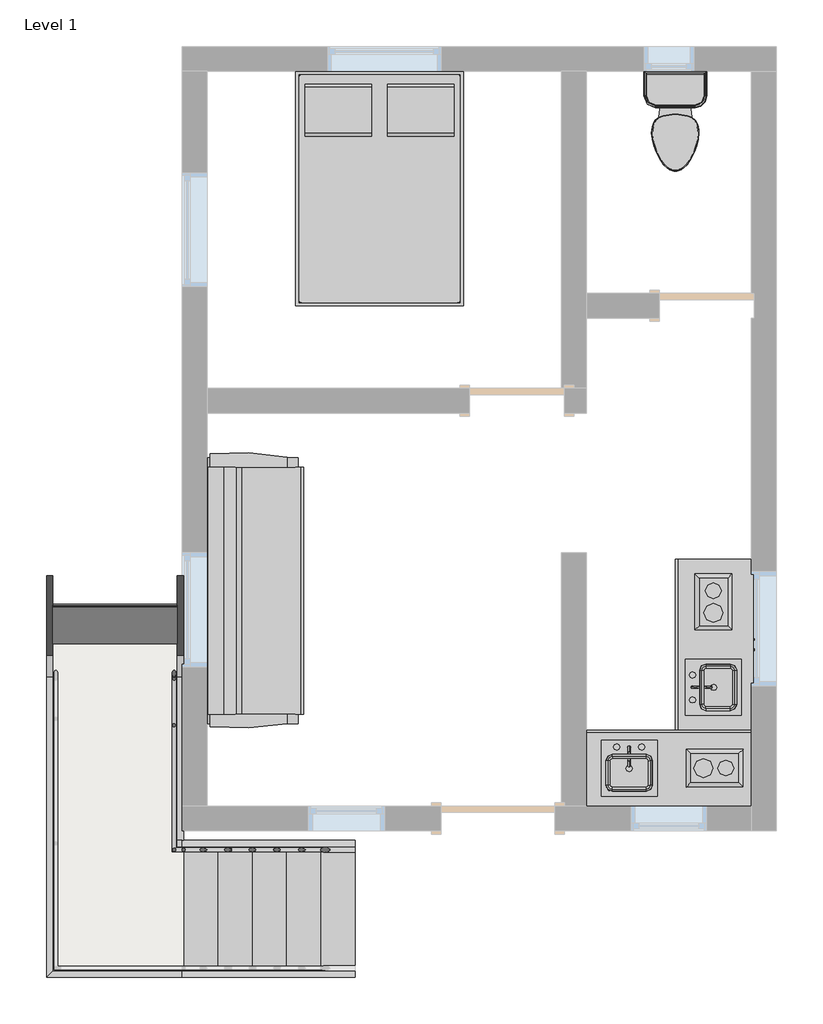
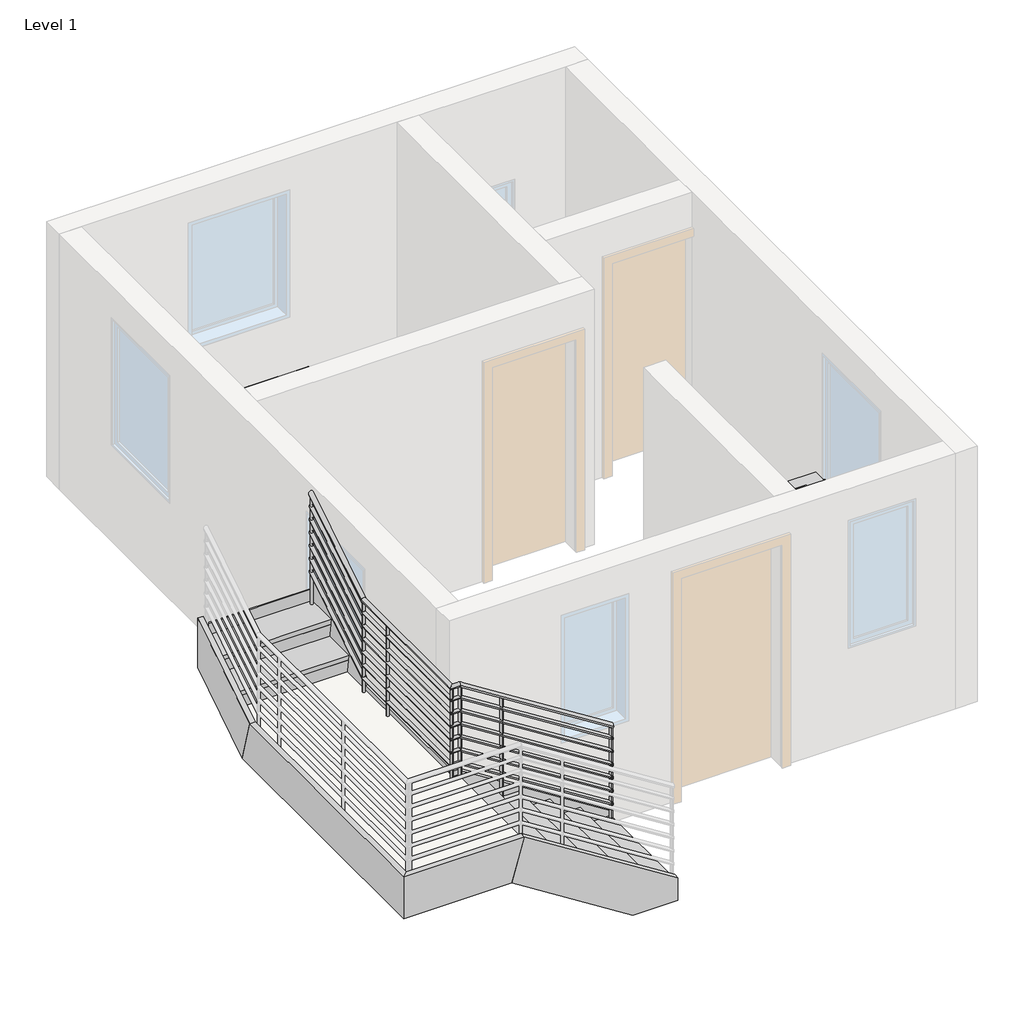
# One storey, part 3 of 3: 7 members, 4 furniture elements, 4 proxies, 3 flow terminals, 2 stair flights, 1 railing, 1 slab.
"""IFC4 building model written with IfcOpenShell, lengths in millimetres."""

from ifc_helpers import new_model, si_unit, point, frame, frame_2d, origin, place, context, project, spatial, polyline, circle_curve, ellipse_curve, trimmed, segment, composite_curve, outline, extrude, faceted_brep, transform, mapped, element, save
from ifc_brep_helpers import plane_surface, cylinder_surface, advanced_brep
from components import m_cook_top_2_unit_305_x_457mm_ebea1746, m_kitchenette_small_1372mm_f81b7602, m_sink_kitchen_island_450_x_450mm_f969cf2d, m_toilet_domestic_3d_m_toilet_domestic_3d_5cb52bd4, m_toilet_domestic_3d_m_toilet_domestic_3d_183bbd19, m_bed_box_1346_x_1880mm_double_b32eb57e, m_counter_top_w_sink_hole_600mm_depth_edbb3572, m_sofa_pensi_2134mm_91f3548c, non_monolithic_landing_de183352, stair_flight_50mm_tread_25mm_nosing_13mm_riser_1fd5534d, stair_flight_50mm_tread_25mm_nosing_13mm_riser_775a8025

model = new_model("IFC4")

# Units and contexts
model_context = context("Model", 3, world=origin())
ifc_project = project(units=[si_unit("LENGTHUNIT", "METRE", prefix="MILLI")], contexts=[model_context])

# Site, building, storey
site = spatial("IfcSite", under=ifc_project)
building = spatial("IfcBuilding", under=site)
storey = spatial("IfcBuildingStorey", under=building, Name="Level 1", Elevation=0.0)

# Proxies
placement = place(None, origin())
m_cook_top_2_unit_305_x_457mm_shape = m_cook_top_2_unit_305_x_457mm_ebea1746(model_context)
element("IfcBuildingElementProxy", 1, Name="M_Cook Top-2 Unit : 305 x 457mm", ObjectType="M_Cook Top-2 Unit : 305 x 457mm", at=placement, inside=storey, context=model_context, shape_type="MappedRepresentation", body=[
    mapped(m_cook_top_2_unit_305_x_457mm_shape, transform((-7256.3238606, 6264.0835626, 40.0), x_axis=(0.0, 1.0, 0.0), y_axis=(-1.0, 0.0, 0.0), z_axis=(0.0, 0.0, 1.0))),
])
element("IfcBuildingElementProxy", 2, Name="M_Cook Top-2 Unit : 305 x 457mm", ObjectType="M_Cook Top-2 Unit : 305 x 457mm", at=placement, inside=storey, context=model_context, shape_type="MappedRepresentation", body=[
    mapped(m_cook_top_2_unit_305_x_457mm_shape, transform((-7220.3486562, 7704.5083582, 40.0), x_axis=(-1.0000000000000002, 0.0, 0.0), y_axis=(0.0, -1.0000000000000002, 0.0), z_axis=(0.0, 0.0, 1.0))),
])
m_kitchenette_small_1372mm_shape = m_kitchenette_small_1372mm_f81b7602(model_context)
element("IfcBuildingElementProxy", 3, Name="M_Kitchenette - Small : 1372mm", ObjectType="M_Kitchenette - Small : 1372mm", at=placement, inside=storey, context=model_context, shape_type="MappedRepresentation", body=[
    mapped(m_kitchenette_small_1372mm_shape, transform((-7648.2863611, 6645.2835626, 0.0), x_axis=(1.0, 0.0, 0.0), y_axis=(0.0, 1.0, 0.0), z_axis=(0.0, 0.0, 1.0))),
])
element("IfcBuildingElementProxy", 4, Name="M_Kitchenette - Small : 1372mm", ObjectType="M_Kitchenette - Small : 1372mm", at=placement, inside=storey, context=model_context, shape_type="MappedRepresentation", body=[
    mapped(m_kitchenette_small_1372mm_shape, transform((-7601.5486562, 7312.5458577, 0.0), x_axis=(0.0, 1.0000000000000002, 0.0), y_axis=(-1.0000000000000002, 0.0, 0.0), z_axis=(0.0, 0.0, 1.0))),
])

# Flow terminals
m_sink_kitchen_island_450_x_450mm_shape = m_sink_kitchen_island_450_x_450mm_f969cf2d(model_context)
element("IfcFlowTerminal", 5, ObjectType="M_Sink Kitchen-Island : 450 x 450mm", at=placement, inside=storey, context=model_context, shape_type="MappedRepresentation", body=[
    mapped(m_sink_kitchen_island_450_x_450mm_shape, transform((-7988.2378968, 6337.9381615, 40.0), x_axis=(1.0, 0.0, 0.0), y_axis=(0.0, 1.0, 0.0), z_axis=(0.0, 0.0, 1.0))),
])
element("IfcFlowTerminal", 6, ObjectType="M_Sink Kitchen-Island : 450 x 450mm", at=placement, inside=storey, context=model_context, shape_type="MappedRepresentation", body=[
    mapped(m_sink_kitchen_island_450_x_450mm_shape, transform((-7294.2032551, 6972.5943221, 40.0), x_axis=(0.0, 1.0000000000000002, 0.0), y_axis=(-1.0000000000000002, 0.0, 0.0), z_axis=(0.0, 0.0, 1.0))),
])
m_toilet_domestic_3d_m_toilet_domestic_3d_shape = m_toilet_domestic_3d_m_toilet_domestic_3d_5cb52bd4(model_context)
m_toilet_domestic_3d_m_toilet_domestic_3d_2_shape = m_toilet_domestic_3d_m_toilet_domestic_3d_183bbd19(model_context)
element("IfcFlowTerminal", 7, ObjectType="M_Toilet-Domestic-3D : M_Toilet-Domestic-3D", at=placement, inside=storey, context=model_context, shape_type="MappedRepresentation", body=[
    mapped(m_toilet_domestic_3d_m_toilet_domestic_3d_shape, transform((-7602.1446836, 11436.5875353, 0.0), x_axis=(1.0, 0.0, 0.0), y_axis=(0.0, 1.0, 0.0), z_axis=(0.0, 0.0, 1.0))),
    mapped(m_toilet_domestic_3d_m_toilet_domestic_3d_2_shape, transform((-7602.1446836, 11436.5875353, 0.0), x_axis=(1.0, 0.0, 0.0), y_axis=(0.0, 1.0, 0.0), z_axis=(0.0, 0.0, 1.0))),
])

# Furniture
m_bed_box_1346_x_1880mm_double_shape = m_bed_box_1346_x_1880mm_double_b32eb57e(model_context)
element("IfcFurniture", 8, ObjectType="M_Bed-Box : 1346 x 1880mm - Double", at=placement, inside=storey, context=model_context, shape_type="MappedRepresentation", body=[
    mapped(m_bed_box_1346_x_1880mm_double_shape, transform((-10316.7011152, 11225.7130708, 0.0), x_axis=(1.0, 0.0, 0.0), y_axis=(0.0, 1.0, 0.0), z_axis=(0.0, 0.0, 1.0))),
])
m_counter_top_w_sink_hole_600mm_depth_shape = m_counter_top_w_sink_hole_600mm_depth_edbb3572(model_context)
element("IfcFurniture", 9, ObjectType="M_Counter Top w Sink Hole : 600mm Depth", at=placement, inside=storey, context=model_context, shape_type="MappedRepresentation", body=[
    mapped(m_counter_top_w_sink_hole_600mm_depth_shape, transform((-7115.0863611, 6645.2835626, 40.0), x_axis=(1.0, 0.0, 0.0), y_axis=(0.0, 1.0, 0.0), z_axis=(0.0, 0.0, 1.0))),
])
element("IfcFurniture", 10, ObjectType="M_Counter Top w Sink Hole : 600mm Depth", at=placement, inside=storey, context=model_context, shape_type="MappedRepresentation", body=[
    mapped(m_counter_top_w_sink_hole_600mm_depth_shape, transform((-7601.5486562, 7845.7458577, 40.0), x_axis=(0.0, 1.0000000000000002, 0.0), y_axis=(-1.0000000000000002, 0.0, 0.0), z_axis=(0.0, 0.0, 1.0))),
])
m_sofa_pensi_2134mm_shape = m_sofa_pensi_2134mm_91f3548c(model_context)
element("IfcFurniture", 11, ObjectType="M_Sofa-Pensi : 2134mm", at=placement, inside=storey, context=model_context, shape_type="MappedRepresentation", body=[
    mapped(m_sofa_pensi_2134mm_shape, transform((-10729.2388201, 7485.4773126, 0.0), x_axis=(0.0, 1.0, 0.0), y_axis=(-1.0, 0.0, 0.0), z_axis=(0.0, 0.0, 1.0))),
])

# Members
element("IfcMember", 12, ObjectType="Stringer - 50mm Width", at=placement, inside=storey, context=model_context, shape_type="SweptSolid", body=[
    extrude(outline(polyline([(0.0, -10176.2529994), (215.089535, -10176.2529994), (1090.8719878, -11561.084003), (690.8719878, -11676.953063), (0.0, -10584.5117322), (0.0, -10176.2529994)])), frame((0.0, 4659.8403022, 0.0), z_axis=(0.0, 1.0, 0.0), x_axis=(0.0, 0.0, 1.0)), (0.0, 0.0, 1.0), 50.0),
])
element("IfcMember", 13, ObjectType="Stringer - 50mm Width", at=placement, inside=storey, context=model_context, shape_type="SweptSolid", body=[
    extrude(outline(polyline([(0.0, -10176.2529994), (215.089535, -10176.2529994), (1090.8719878, -11561.084003), (1090.8719878, -11602.0529994), (643.5043587, -11602.0529994), (0.0, -10584.5117322), (0.0, -10176.2529994)])), frame((0.0, 5709.8660835, 0.0), z_axis=(0.0, 1.0, 0.0), x_axis=(0.0, 0.0, 1.0)), (0.0, 0.0, 1.0), 50.0),
])
element("IfcMember", 14, ObjectType="Stringer - 50mm Width", at=placement, inside=storey, context=model_context, shape_type="SweptSolid", body=[
    extrude(outline(polyline([(7184.5661471, 690.8719878), (7068.697087, 1090.8719878), (7883.8660835, 1606.3938828), (7883.8660835, 1133.1170069), (7184.5661471, 690.8719878)])), frame((-12652.0787807, 0.0, 0.0), z_axis=(1.0, 0.0, 0.0), x_axis=(0.0, 1.0, 0.0)), (0.0, 0.0, 1.0), 50.0),
])
element("IfcMember", 15, ObjectType="Stringer - 50mm Width", at=placement, inside=storey, context=model_context, shape_type="SweptSolid", body=[
    extrude(outline(polyline([(7184.5661471, 690.8719878), (7068.697087, 1090.8719878), (7883.8660835, 1606.3938828), (7883.8660835, 1133.1170069), (7184.5661471, 690.8719878)])), frame((-11602.0529994, 0.0, 0.0), z_axis=(1.0, 0.0, 0.0), x_axis=(0.0, 1.0, 0.0)), (0.0, 0.0, 1.0), 50.0),
])
element("IfcMember", 16, ObjectType="Stringer - 50mm Width", at=placement, inside=storey, context=model_context, shape_type="Brep", body=[
    faceted_brep([(-12602.0787807, 7068.697087, 1090.8719878), (-12652.0787807, 7068.697087, 1090.8719878), (-12652.0787807, 4659.8403022, 1090.8719878), (-12602.0787807, 4709.8403022, 1090.8719878), (-12602.0787807, 7184.5661471, 690.8719878), (-12602.0787807, 4709.8403022, 690.8719878), (-12652.0787807, 7184.5661471, 690.8719878), (-12652.0787807, 4659.8403022, 690.8719878)], [[[0, 1, 2, 3]], [[4, 0, 3, 5]], [[6, 4, 5, 7]], [[1, 6, 7, 2]], [[1, 0, 4, 6]], [[2, 7, 5, 3]]]),
])
element("IfcMember", 17, ObjectType="Stringer - 50mm Width", at=placement, inside=storey, context=model_context, shape_type="Brep", body=[
    faceted_brep([(-12602.0787807, 4709.8403022, 1090.8719878), (-12652.0787807, 4659.8403022, 1090.8719878), (-11561.084003, 4659.8403022, 1090.8719878), (-11561.084003, 4709.8403022, 1090.8719878), (-12602.0787807, 4709.8403022, 690.8719878), (-11676.953063, 4709.8403022, 690.8719878), (-12652.0787807, 4659.8403022, 690.8719878), (-11676.953063, 4659.8403022, 690.8719878)], [[[0, 1, 2, 3]], [[4, 0, 3, 5]], [[6, 4, 5, 7]], [[1, 6, 7, 2]], [[1, 0, 4, 6]], [[2, 7, 5, 3]]]),
])
element("IfcMember", 18, ObjectType="Stringer - 50mm Width", at=placement, inside=storey, context=model_context, shape_type="SweptSolid", body=[
    extrude(outline(polyline([(5759.8660835, 690.8719878), (5759.8660835, 1090.8719878), (7068.697087, 1090.8719878), (7184.5661471, 690.8719878), (5759.8660835, 690.8719878)])), frame((-11602.0529994, 0.0, 0.0), z_axis=(1.0, 0.0, 0.0), x_axis=(0.0, 1.0, 0.0)), (0.0, 0.0, 1.0), 50.0),
])

# Railing
element("IfcRailing", 19, ObjectType="900mm Pipe", at=placement, inside=storey, context=model_context, shape_type="SolidModel", body=[
    advanced_brep(
    [(-10176.2529994, 5704.4660835, 1050.2491997), (-10176.2529994, 5664.4660835, 1050.2491997), (-11557.0464524, 5704.4660835, 1923.4782609), (-11557.0464524, 5664.4660835, 1923.4782609), (-11607.4529994, 5704.4660835, 1923.4782609), (-11647.4529994, 5664.4660835, 1923.4782609), (-11607.4529994, 7064.6595365, 1923.4782609), (-11647.4529994, 7064.6595365, 1923.4782609), (-11607.4529994, 7883.8660835, 2441.5535475), (-11647.4529994, 7883.8660835, 2441.5535475)],
    [
        (0, 1, ellipse_curve(frame((-10176.2529994, 5684.4660835, 1050.2491997), z_axis=(1.0, 0.0, 0.0), x_axis=(0.0, 0.0, -1.0)), 23.6638438, 20.0)),
        (1, 0, ellipse_curve(frame((-10176.2529994, 5684.4660835, 1050.2491997), z_axis=(1.0, 0.0, 0.0), x_axis=(0.0, 0.0, -1.0)), 23.6638438, 20.0)),
        (0, 2),
        (2, 3, ellipse_curve(frame((-11557.0464524, 5684.4660835, 1923.4782609), z_axis=(0.9605132043335073, 0.0, -0.2782344053149754), x_axis=(-0.278234405314975, 0.0, -0.9605132043335074)), 20.822202, 20.0)),
        (3, 1),
        (3, 2, ellipse_curve(frame((-11557.0464524, 5684.4660835, 1923.4782609), z_axis=(0.9605132043335073, 0.0, -0.2782344053149754), x_axis=(-0.278234405314975, 0.0, -0.9605132043335074)), 20.822202, 20.0)),
        (2, 4),
        (4, 5, ellipse_curve(frame((-11627.4529994, 5684.4660835, 1923.4782609), z_axis=(0.7071067811865452, -0.7071067811865499, 0.0), x_axis=(0.7071067811865497, 0.7071067811865452, 0.0)), 28.2842712, 20.0)),
        (5, 3),
        (5, 4, ellipse_curve(frame((-11627.4529994, 5684.4660835, 1923.4782609), z_axis=(0.7071067811865452, -0.7071067811865499, 0.0), x_axis=(0.7071067811865497, 0.7071067811865452, 0.0)), 28.2842712, 20.0)),
        (4, 6),
        (6, 7, ellipse_curve(frame((-11627.4529994, 7064.6595365, 1923.4782609), z_axis=(0.0, -0.9605132043335063, -0.27823440531497884), x_axis=(0.0, -0.2782344053149792, 0.9605132043335064)), 20.822202, 20.0)),
        (7, 5),
        (7, 6, ellipse_curve(frame((-11627.4529994, 7064.6595365, 1923.4782609), z_axis=(0.0, -0.9605132043335063, -0.27823440531497884), x_axis=(0.0, -0.2782344053149792, 0.9605132043335064)), 20.822202, 20.0)),
        (8, 9, ellipse_curve(frame((-11627.4529994, 7883.8660835, 2441.5535475), z_axis=(0.0, 1.0, 0.0), x_axis=(0.0, 0.0, -1.0)), 23.6638438, 20.0)),
        (9, 8, ellipse_curve(frame((-11627.4529994, 7883.8660835, 2441.5535475), z_axis=(0.0, 1.0, 0.0), x_axis=(0.0, 0.0, -1.0)), 23.6638438, 20.0)),
        (6, 8),
        (9, 7),
    ],
    [
        plane_surface(frame((-10176.2529994, 5684.4660835, 1073.9130435), z_axis=(1.0, 0.0, 0.0), x_axis=(0.0, -1.0, 0.0))),
        cylinder_surface(frame((-10186.9429122, 5684.4660835, 1057.0096189), z_axis=(0.845171231398044, 0.0, -0.5344956404098298), x_axis=(0.0, -1.0, 0.0)), 20.0),
        cylinder_surface(frame((-11551.2529994, 5684.4660835, 1923.4782609), z_axis=(1.0, 0.0, 0.0), x_axis=(0.0, -1.0, 0.0)), 20.0),
        cylinder_surface(frame((-11627.4529994, 5684.4660835, 1923.4782609), z_axis=(0.0, -1.0, 0.0), x_axis=(-1.0, 0.0, 0.0)), 20.0),
        plane_surface(frame((-11627.4529994, 7883.8660835, 2465.2173913), z_axis=(0.0, 1.0, 0.0), x_axis=(0.0, 0.0, 1.0))),
        cylinder_surface(frame((-11627.4529994, 7069.5559963, 1926.5748362), z_axis=(0.0, -0.8451712313980402, -0.5344956404098358), x_axis=(-1.0, 0.0, 0.0)), 20.0),
    ],
    [
        (0, [[1, 2]]),
        (1, [[-1, 3, 4, 5]]),
        (1, [[-2, -5, 6, -3]]),
        (2, [[-4, 7, 8, 9]]),
        (2, [[-6, -9, 10, -7]]),
        (3, [[-8, 11, 12, 13]]),
        (3, [[-10, -13, 14, -11]]),
        (4, [[15, 16]]),
        (5, [[-12, 17, -16, 18]]),
        (5, [[-14, -18, -15, -17]]),
    ],
),
    advanced_brep(
    [(-10176.2529994, 5669.4660835, 931.1651606), (-10176.2529994, 5699.4660835, 931.1651606), (-11555.5980892, 5669.4660835, 1803.4782609), (-11555.5980892, 5699.4660835, 1803.4782609), (-11642.4529994, 5669.4660835, 1803.4782609), (-11612.4529994, 5699.4660835, 1803.4782609), (-11642.4529994, 7063.2111733, 1803.4782609), (-11612.4529994, 7063.2111733, 1803.4782609), (-11642.4529994, 7883.8660835, 2322.4695085), (-11612.4529994, 7883.8660835, 2322.4695085)],
    [
        (0, 1, ellipse_curve(frame((-10176.2529994, 5684.4660835, 931.1651606), z_axis=(1.0, 0.0, 0.0), x_axis=(0.0, 0.0, -1.0)), 17.7478828, 15.0)),
        (1, 0, ellipse_curve(frame((-10176.2529994, 5684.4660835, 931.1651606), z_axis=(1.0, 0.0, 0.0), x_axis=(0.0, 0.0, -1.0)), 17.7478828, 15.0)),
        (0, 2),
        (2, 3, ellipse_curve(frame((-11555.5980892, 5684.4660835, 1803.4782609), z_axis=(0.9605132043335073, 0.0, -0.27823440531497534), x_axis=(-0.27823440531497506, 0.0, -0.9605132043335075)), 15.6166515, 15.0)),
        (3, 1),
        (3, 2, ellipse_curve(frame((-11555.5980892, 5684.4660835, 1803.4782609), z_axis=(0.9605132043335073, 0.0, -0.27823440531497534), x_axis=(-0.27823440531497506, 0.0, -0.9605132043335075)), 15.6166515, 15.0)),
        (2, 4),
        (4, 5, ellipse_curve(frame((-11627.4529994, 5684.4660835, 1803.4782609), z_axis=(0.7071067811865452, -0.7071067811865499, 0.0), x_axis=(0.7071067811865497, 0.7071067811865452, 0.0)), 21.2132034, 15.0)),
        (5, 3),
        (5, 4, ellipse_curve(frame((-11627.4529994, 5684.4660835, 1803.4782609), z_axis=(0.7071067811865452, -0.7071067811865499, 0.0), x_axis=(0.7071067811865497, 0.7071067811865452, 0.0)), 21.2132034, 15.0)),
        (4, 6),
        (6, 7, ellipse_curve(frame((-11627.4529994, 7063.2111733, 1803.4782609), z_axis=(0.0, -0.9605132043335064, -0.2782344053149787), x_axis=(0.0, -0.27823440531497856, 0.9605132043335064)), 15.6166515, 15.0)),
        (7, 5),
        (7, 6, ellipse_curve(frame((-11627.4529994, 7063.2111733, 1803.4782609), z_axis=(0.0, -0.9605132043335064, -0.2782344053149787), x_axis=(0.0, -0.27823440531497856, 0.9605132043335064)), 15.6166515, 15.0)),
        (8, 9, ellipse_curve(frame((-11627.4529994, 7883.8660835, 2322.4695085), z_axis=(0.0, 1.0, 0.0), x_axis=(0.0, 0.0, -1.0)), 17.7478828, 15.0)),
        (9, 8, ellipse_curve(frame((-11627.4529994, 7883.8660835, 2322.4695085), z_axis=(0.0, 1.0, 0.0), x_axis=(0.0, 0.0, -1.0)), 17.7478828, 15.0)),
        (6, 8),
        (9, 7),
    ],
    [
        plane_surface(frame((-10176.2529994, 5684.4660835, 948.9130435), z_axis=(1.0, 0.0, 0.0), x_axis=(0.0, -1.0, 0.0))),
        cylinder_surface(frame((-10184.270434, 5684.4660835, 936.235475), z_axis=(0.845171231398044, 0.0, -0.5344956404098297), x_axis=(0.0, 1.0, 0.0)), 15.0),
        cylinder_surface(frame((-11551.2529994, 5684.4660835, 1803.4782609), z_axis=(1.0, 0.0, 0.0), x_axis=(0.0, 1.0, 0.0)), 15.0),
        cylinder_surface(frame((-11627.4529994, 5684.4660835, 1803.4782609), z_axis=(0.0, -1.0, 0.0), x_axis=(1.0, 0.0, 0.0)), 15.0),
        plane_surface(frame((-11627.4529994, 7883.8660835, 2340.2173913), z_axis=(0.0, 1.0, 0.0), x_axis=(0.0, 0.0, 1.0))),
        cylinder_surface(frame((-11627.4529994, 7066.8835181, 1805.8006924), z_axis=(0.0, -0.8451712313980403, -0.5344956404098355), x_axis=(1.0, 0.0, 0.0)), 15.0),
    ],
    [
        (0, [[1, 2]]),
        (1, [[-1, 3, 4, 5]]),
        (1, [[-2, -5, 6, -3]]),
        (2, [[-4, 7, 8, 9]]),
        (2, [[-6, -9, 10, -7]]),
        (3, [[-8, 11, 12, 13]]),
        (3, [[-10, -13, 14, -11]]),
        (4, [[15, 16]]),
        (5, [[-12, 17, -16, 18]]),
        (5, [[-14, -18, -15, -17]]),
    ],
),
    advanced_brep(
    [(-10176.2529994, 5669.4660835, 806.1651606), (-10176.2529994, 5699.4660835, 806.1651606), (-11555.5980892, 5669.4660835, 1678.4782609), (-11555.5980892, 5699.4660835, 1678.4782609), (-11642.4529994, 5669.4660835, 1678.4782609), (-11612.4529994, 5699.4660835, 1678.4782609), (-11642.4529994, 7063.2111733, 1678.4782609), (-11612.4529994, 7063.2111733, 1678.4782609), (-11642.4529994, 7883.8660835, 2197.4695085), (-11612.4529994, 7883.8660835, 2197.4695085)],
    [
        (0, 1, ellipse_curve(frame((-10176.2529994, 5684.4660835, 806.1651606), z_axis=(1.0, 0.0, 0.0), x_axis=(0.0, 0.0, -1.0)), 17.7478828, 15.0)),
        (1, 0, ellipse_curve(frame((-10176.2529994, 5684.4660835, 806.1651606), z_axis=(1.0, 0.0, 0.0), x_axis=(0.0, 0.0, -1.0)), 17.7478828, 15.0)),
        (0, 2),
        (2, 3, ellipse_curve(frame((-11555.5980892, 5684.4660835, 1678.4782609), z_axis=(0.9605132043335073, 0.0, -0.27823440531497534), x_axis=(-0.27823440531497506, 0.0, -0.9605132043335075)), 15.6166515, 15.0)),
        (3, 1),
        (3, 2, ellipse_curve(frame((-11555.5980892, 5684.4660835, 1678.4782609), z_axis=(0.9605132043335073, 0.0, -0.27823440531497534), x_axis=(-0.27823440531497506, 0.0, -0.9605132043335075)), 15.6166515, 15.0)),
        (2, 4),
        (4, 5, ellipse_curve(frame((-11627.4529994, 5684.4660835, 1678.4782609), z_axis=(0.7071067811865452, -0.7071067811865499, 0.0), x_axis=(0.7071067811865497, 0.7071067811865452, 0.0)), 21.2132034, 15.0)),
        (5, 3),
        (5, 4, ellipse_curve(frame((-11627.4529994, 5684.4660835, 1678.4782609), z_axis=(0.7071067811865452, -0.7071067811865499, 0.0), x_axis=(0.7071067811865497, 0.7071067811865452, 0.0)), 21.2132034, 15.0)),
        (4, 6),
        (6, 7, ellipse_curve(frame((-11627.4529994, 7063.2111733, 1678.4782609), z_axis=(0.0, -0.9605132043335063, -0.27823440531497884), x_axis=(0.0, -0.2782344053149792, 0.9605132043335064)), 15.6166515, 15.0)),
        (7, 5),
        (7, 6, ellipse_curve(frame((-11627.4529994, 7063.2111733, 1678.4782609), z_axis=(0.0, -0.9605132043335063, -0.27823440531497884), x_axis=(0.0, -0.2782344053149792, 0.9605132043335064)), 15.6166515, 15.0)),
        (8, 9, ellipse_curve(frame((-11627.4529994, 7883.8660835, 2197.4695085), z_axis=(0.0, 1.0, 0.0), x_axis=(0.0, 0.0, -1.0)), 17.7478828, 15.0)),
        (9, 8, ellipse_curve(frame((-11627.4529994, 7883.8660835, 2197.4695085), z_axis=(0.0, 1.0, 0.0), x_axis=(0.0, 0.0, -1.0)), 17.7478828, 15.0)),
        (6, 8),
        (9, 7),
    ],
    [
        plane_surface(frame((-10176.2529994, 5684.4660835, 823.9130435), z_axis=(1.0, 0.0, 0.0), x_axis=(0.0, -1.0, 0.0))),
        cylinder_surface(frame((-10184.270434, 5684.4660835, 811.235475), z_axis=(0.845171231398044, 0.0, -0.5344956404098297), x_axis=(0.0, 1.0, 0.0)), 15.0),
        cylinder_surface(frame((-11551.2529994, 5684.4660835, 1678.4782609), z_axis=(1.0, 0.0, 0.0), x_axis=(0.0, 1.0, 0.0)), 15.0),
        cylinder_surface(frame((-11627.4529994, 5684.4660835, 1678.4782609), z_axis=(0.0, -1.0, 0.0), x_axis=(1.0, 0.0, 0.0)), 15.0),
        plane_surface(frame((-11627.4529994, 7883.8660835, 2215.2173913), z_axis=(0.0, 1.0, 0.0), x_axis=(0.0, 0.0, 1.0))),
        cylinder_surface(frame((-11627.4529994, 7066.8835181, 1680.8006924), z_axis=(0.0, -0.8451712313980402, -0.5344956404098358), x_axis=(1.0, 0.0, 0.0)), 15.0),
    ],
    [
        (0, [[1, 2]]),
        (1, [[-1, 3, 4, 5]]),
        (1, [[-2, -5, 6, -3]]),
        (2, [[-4, 7, 8, 9]]),
        (2, [[-6, -9, 10, -7]]),
        (3, [[-8, 11, 12, 13]]),
        (3, [[-10, -13, 14, -11]]),
        (4, [[15, 16]]),
        (5, [[-12, 17, -16, 18]]),
        (5, [[-14, -18, -15, -17]]),
    ],
),
    advanced_brep(
    [(-10176.2529994, 5669.4660835, 681.1651606), (-10176.2529994, 5699.4660835, 681.1651606), (-11555.5980892, 5669.4660835, 1553.4782609), (-11555.5980892, 5699.4660835, 1553.4782609), (-11642.4529994, 5669.4660835, 1553.4782609), (-11612.4529994, 5699.4660835, 1553.4782609), (-11642.4529994, 7063.2111733, 1553.4782609), (-11612.4529994, 7063.2111733, 1553.4782609), (-11642.4529994, 7883.8660835, 2072.4695085), (-11612.4529994, 7883.8660835, 2072.4695085)],
    [
        (0, 1, ellipse_curve(frame((-10176.2529994, 5684.4660835, 681.1651606), z_axis=(1.0, 0.0, 0.0), x_axis=(0.0, 0.0, -1.0)), 17.7478828, 15.0)),
        (1, 0, ellipse_curve(frame((-10176.2529994, 5684.4660835, 681.1651606), z_axis=(1.0, 0.0, 0.0), x_axis=(0.0, 0.0, -1.0)), 17.7478828, 15.0)),
        (0, 2),
        (2, 3, ellipse_curve(frame((-11555.5980892, 5684.4660835, 1553.4782609), z_axis=(0.9605132043335073, 0.0, -0.27823440531497534), x_axis=(-0.27823440531497506, 0.0, -0.9605132043335075)), 15.6166515, 15.0)),
        (3, 1),
        (3, 2, ellipse_curve(frame((-11555.5980892, 5684.4660835, 1553.4782609), z_axis=(0.9605132043335073, 0.0, -0.27823440531497534), x_axis=(-0.27823440531497506, 0.0, -0.9605132043335075)), 15.6166515, 15.0)),
        (2, 4),
        (4, 5, ellipse_curve(frame((-11627.4529994, 5684.4660835, 1553.4782609), z_axis=(0.7071067811865452, -0.7071067811865499, 0.0), x_axis=(0.7071067811865497, 0.7071067811865452, 0.0)), 21.2132034, 15.0)),
        (5, 3),
        (5, 4, ellipse_curve(frame((-11627.4529994, 5684.4660835, 1553.4782609), z_axis=(0.7071067811865452, -0.7071067811865499, 0.0), x_axis=(0.7071067811865497, 0.7071067811865452, 0.0)), 21.2132034, 15.0)),
        (4, 6),
        (6, 7, ellipse_curve(frame((-11627.4529994, 7063.2111733, 1553.4782609), z_axis=(0.0, -0.9605132043335064, -0.2782344053149787), x_axis=(0.0, -0.27823440531497856, 0.9605132043335064)), 15.6166515, 15.0)),
        (7, 5),
        (7, 6, ellipse_curve(frame((-11627.4529994, 7063.2111733, 1553.4782609), z_axis=(0.0, -0.9605132043335064, -0.2782344053149787), x_axis=(0.0, -0.27823440531497856, 0.9605132043335064)), 15.6166515, 15.0)),
        (8, 9, ellipse_curve(frame((-11627.4529994, 7883.8660835, 2072.4695085), z_axis=(0.0, 1.0, 0.0), x_axis=(0.0, 0.0, -1.0)), 17.7478828, 15.0)),
        (9, 8, ellipse_curve(frame((-11627.4529994, 7883.8660835, 2072.4695085), z_axis=(0.0, 1.0, 0.0), x_axis=(0.0, 0.0, -1.0)), 17.7478828, 15.0)),
        (6, 8),
        (9, 7),
    ],
    [
        plane_surface(frame((-10176.2529994, 5684.4660835, 698.9130435), z_axis=(1.0, 0.0, 0.0), x_axis=(0.0, -1.0, 0.0))),
        cylinder_surface(frame((-10184.270434, 5684.4660835, 686.235475), z_axis=(0.845171231398044, 0.0, -0.5344956404098297), x_axis=(0.0, 1.0, 0.0)), 15.0),
        cylinder_surface(frame((-11551.2529994, 5684.4660835, 1553.4782609), z_axis=(1.0, 0.0, 0.0), x_axis=(0.0, 1.0, 0.0)), 15.0),
        cylinder_surface(frame((-11627.4529994, 5684.4660835, 1553.4782609), z_axis=(0.0, -1.0, 0.0), x_axis=(1.0, 0.0, 0.0)), 15.0),
        plane_surface(frame((-11627.4529994, 7883.8660835, 2090.2173913), z_axis=(0.0, 1.0, 0.0), x_axis=(0.0, 0.0, 1.0))),
        cylinder_surface(frame((-11627.4529994, 7066.8835181, 1555.8006924), z_axis=(0.0, -0.8451712313980403, -0.5344956404098355), x_axis=(1.0, 0.0, 0.0)), 15.0),
    ],
    [
        (0, [[1, 2]]),
        (1, [[-1, 3, 4, 5]]),
        (1, [[-2, -5, 6, -3]]),
        (2, [[-4, 7, 8, 9]]),
        (2, [[-6, -9, 10, -7]]),
        (3, [[-8, 11, 12, 13]]),
        (3, [[-10, -13, 14, -11]]),
        (4, [[15, 16]]),
        (5, [[-12, 17, -16, 18]]),
        (5, [[-14, -18, -15, -17]]),
    ],
),
    advanced_brep(
    [(-10176.2529994, 5669.4660835, 556.1651606), (-10176.2529994, 5699.4660835, 556.1651606), (-11555.5980892, 5669.4660835, 1428.4782609), (-11555.5980892, 5699.4660835, 1428.4782609), (-11642.4529994, 5669.4660835, 1428.4782609), (-11612.4529994, 5699.4660835, 1428.4782609), (-11642.4529994, 7063.2111733, 1428.4782609), (-11612.4529994, 7063.2111733, 1428.4782609), (-11642.4529994, 7883.8660835, 1947.4695085), (-11612.4529994, 7883.8660835, 1947.4695085)],
    [
        (0, 1, ellipse_curve(frame((-10176.2529994, 5684.4660835, 556.1651606), z_axis=(1.0, 0.0, 0.0), x_axis=(0.0, 0.0, -1.0)), 17.7478828, 15.0)),
        (1, 0, ellipse_curve(frame((-10176.2529994, 5684.4660835, 556.1651606), z_axis=(1.0, 0.0, 0.0), x_axis=(0.0, 0.0, -1.0)), 17.7478828, 15.0)),
        (0, 2),
        (2, 3, ellipse_curve(frame((-11555.5980892, 5684.4660835, 1428.4782609), z_axis=(0.9605132043335073, 0.0, -0.27823440531497534), x_axis=(-0.27823440531497506, 0.0, -0.9605132043335075)), 15.6166515, 15.0)),
        (3, 1),
        (3, 2, ellipse_curve(frame((-11555.5980892, 5684.4660835, 1428.4782609), z_axis=(0.9605132043335073, 0.0, -0.27823440531497534), x_axis=(-0.27823440531497506, 0.0, -0.9605132043335075)), 15.6166515, 15.0)),
        (2, 4),
        (4, 5, ellipse_curve(frame((-11627.4529994, 5684.4660835, 1428.4782609), z_axis=(0.7071067811865452, -0.7071067811865499, 0.0), x_axis=(0.7071067811865497, 0.7071067811865452, 0.0)), 21.2132034, 15.0)),
        (5, 3),
        (5, 4, ellipse_curve(frame((-11627.4529994, 5684.4660835, 1428.4782609), z_axis=(0.7071067811865452, -0.7071067811865499, 0.0), x_axis=(0.7071067811865497, 0.7071067811865452, 0.0)), 21.2132034, 15.0)),
        (4, 6),
        (6, 7, ellipse_curve(frame((-11627.4529994, 7063.2111733, 1428.4782609), z_axis=(0.0, -0.9605132043335063, -0.27823440531497884), x_axis=(0.0, -0.2782344053149792, 0.9605132043335064)), 15.6166515, 15.0)),
        (7, 5),
        (7, 6, ellipse_curve(frame((-11627.4529994, 7063.2111733, 1428.4782609), z_axis=(0.0, -0.9605132043335063, -0.27823440531497884), x_axis=(0.0, -0.2782344053149792, 0.9605132043335064)), 15.6166515, 15.0)),
        (8, 9, ellipse_curve(frame((-11627.4529994, 7883.8660835, 1947.4695085), z_axis=(0.0, 1.0, 0.0), x_axis=(0.0, 0.0, -1.0)), 17.7478828, 15.0)),
        (9, 8, ellipse_curve(frame((-11627.4529994, 7883.8660835, 1947.4695085), z_axis=(0.0, 1.0, 0.0), x_axis=(0.0, 0.0, -1.0)), 17.7478828, 15.0)),
        (6, 8),
        (9, 7),
    ],
    [
        plane_surface(frame((-10176.2529994, 5684.4660835, 573.9130435), z_axis=(1.0, 0.0, 0.0), x_axis=(0.0, -1.0, 0.0))),
        cylinder_surface(frame((-10184.270434, 5684.4660835, 561.235475), z_axis=(0.845171231398044, 0.0, -0.5344956404098297), x_axis=(0.0, 1.0, 0.0)), 15.0),
        cylinder_surface(frame((-11551.2529994, 5684.4660835, 1428.4782609), z_axis=(1.0, 0.0, 0.0), x_axis=(0.0, 1.0, 0.0)), 15.0),
        cylinder_surface(frame((-11627.4529994, 5684.4660835, 1428.4782609), z_axis=(0.0, -1.0, 0.0), x_axis=(1.0, 0.0, 0.0)), 15.0),
        plane_surface(frame((-11627.4529994, 7883.8660835, 1965.2173913), z_axis=(0.0, 1.0, 0.0), x_axis=(0.0, 0.0, 1.0))),
        cylinder_surface(frame((-11627.4529994, 7066.8835181, 1430.8006924), z_axis=(0.0, -0.8451712313980402, -0.5344956404098358), x_axis=(1.0, 0.0, 0.0)), 15.0),
    ],
    [
        (0, [[1, 2]]),
        (1, [[-1, 3, 4, 5]]),
        (1, [[-2, -5, 6, -3]]),
        (2, [[-4, 7, 8, 9]]),
        (2, [[-6, -9, 10, -7]]),
        (3, [[-8, 11, 12, 13]]),
        (3, [[-10, -13, 14, -11]]),
        (4, [[15, 16]]),
        (5, [[-12, 17, -16, 18]]),
        (5, [[-14, -18, -15, -17]]),
    ],
),
    advanced_brep(
    [(-10176.2529994, 5669.4660835, 431.1651606), (-10176.2529994, 5699.4660835, 431.1651606), (-11555.5980892, 5669.4660835, 1303.4782609), (-11555.5980892, 5699.4660835, 1303.4782609), (-11642.4529994, 5669.4660835, 1303.4782609), (-11612.4529994, 5699.4660835, 1303.4782609), (-11642.4529994, 7063.2111733, 1303.4782609), (-11612.4529994, 7063.2111733, 1303.4782609), (-11642.4529994, 7883.8660835, 1822.4695085), (-11612.4529994, 7883.8660835, 1822.4695085)],
    [
        (0, 1, ellipse_curve(frame((-10176.2529994, 5684.4660835, 431.1651606), z_axis=(1.0, 0.0, 0.0), x_axis=(0.0, 0.0, -1.0)), 17.7478828, 15.0)),
        (1, 0, ellipse_curve(frame((-10176.2529994, 5684.4660835, 431.1651606), z_axis=(1.0, 0.0, 0.0), x_axis=(0.0, 0.0, -1.0)), 17.7478828, 15.0)),
        (0, 2),
        (2, 3, ellipse_curve(frame((-11555.5980892, 5684.4660835, 1303.4782609), z_axis=(0.9605132043335073, 0.0, -0.27823440531497534), x_axis=(-0.27823440531497506, 0.0, -0.9605132043335075)), 15.6166515, 15.0)),
        (3, 1),
        (3, 2, ellipse_curve(frame((-11555.5980892, 5684.4660835, 1303.4782609), z_axis=(0.9605132043335073, 0.0, -0.27823440531497534), x_axis=(-0.27823440531497506, 0.0, -0.9605132043335075)), 15.6166515, 15.0)),
        (2, 4),
        (4, 5, ellipse_curve(frame((-11627.4529994, 5684.4660835, 1303.4782609), z_axis=(0.7071067811865452, -0.7071067811865499, 0.0), x_axis=(0.7071067811865497, 0.7071067811865452, 0.0)), 21.2132034, 15.0)),
        (5, 3),
        (5, 4, ellipse_curve(frame((-11627.4529994, 5684.4660835, 1303.4782609), z_axis=(0.7071067811865452, -0.7071067811865499, 0.0), x_axis=(0.7071067811865497, 0.7071067811865452, 0.0)), 21.2132034, 15.0)),
        (4, 6),
        (6, 7, ellipse_curve(frame((-11627.4529994, 7063.2111733, 1303.4782609), z_axis=(0.0, -0.9605132043335064, -0.2782344053149787), x_axis=(0.0, -0.27823440531497856, 0.9605132043335064)), 15.6166515, 15.0)),
        (7, 5),
        (7, 6, ellipse_curve(frame((-11627.4529994, 7063.2111733, 1303.4782609), z_axis=(0.0, -0.9605132043335064, -0.2782344053149787), x_axis=(0.0, -0.27823440531497856, 0.9605132043335064)), 15.6166515, 15.0)),
        (8, 9, ellipse_curve(frame((-11627.4529994, 7883.8660835, 1822.4695085), z_axis=(0.0, 1.0, 0.0), x_axis=(0.0, 0.0, -1.0)), 17.7478828, 15.0)),
        (9, 8, ellipse_curve(frame((-11627.4529994, 7883.8660835, 1822.4695085), z_axis=(0.0, 1.0, 0.0), x_axis=(0.0, 0.0, -1.0)), 17.7478828, 15.0)),
        (6, 8),
        (9, 7),
    ],
    [
        plane_surface(frame((-10176.2529994, 5684.4660835, 448.9130435), z_axis=(1.0, 0.0, 0.0), x_axis=(0.0, -1.0, 0.0))),
        cylinder_surface(frame((-10184.270434, 5684.4660835, 436.235475), z_axis=(0.845171231398044, 0.0, -0.5344956404098297), x_axis=(0.0, 1.0, 0.0)), 15.0),
        cylinder_surface(frame((-11551.2529994, 5684.4660835, 1303.4782609), z_axis=(1.0, 0.0, 0.0), x_axis=(0.0, 1.0, 0.0)), 15.0),
        cylinder_surface(frame((-11627.4529994, 5684.4660835, 1303.4782609), z_axis=(0.0, -1.0, 0.0), x_axis=(1.0, 0.0, 0.0)), 15.0),
        plane_surface(frame((-11627.4529994, 7883.8660835, 1840.2173913), z_axis=(0.0, 1.0, 0.0), x_axis=(0.0, 0.0, 1.0))),
        cylinder_surface(frame((-11627.4529994, 7066.8835181, 1305.8006924), z_axis=(0.0, -0.8451712313980403, -0.5344956404098355), x_axis=(1.0, 0.0, 0.0)), 15.0),
    ],
    [
        (0, [[1, 2]]),
        (1, [[-1, 3, 4, 5]]),
        (1, [[-2, -5, 6, -3]]),
        (2, [[-4, 7, 8, 9]]),
        (2, [[-6, -9, 10, -7]]),
        (3, [[-8, 11, 12, 13]]),
        (3, [[-10, -13, 14, -11]]),
        (4, [[15, 16]]),
        (5, [[-12, 17, -16, 18]]),
        (5, [[-14, -18, -15, -17]]),
    ],
),
    advanced_brep(
    [(-10176.2529994, 5669.4660835, 306.1651606), (-10176.2529994, 5699.4660835, 306.1651606), (-11555.5980892, 5669.4660835, 1178.4782609), (-11555.5980892, 5699.4660835, 1178.4782609), (-11642.4529994, 5669.4660835, 1178.4782609), (-11612.4529994, 5699.4660835, 1178.4782609), (-11642.4529994, 7063.2111733, 1178.4782609), (-11612.4529994, 7063.2111733, 1178.4782609), (-11642.4529994, 7883.8660835, 1697.4695085), (-11612.4529994, 7883.8660835, 1697.4695085)],
    [
        (0, 1, ellipse_curve(frame((-10176.2529994, 5684.4660835, 306.1651606), z_axis=(1.0, 0.0, 0.0), x_axis=(0.0, 0.0, -1.0)), 17.7478828, 15.0)),
        (1, 0, ellipse_curve(frame((-10176.2529994, 5684.4660835, 306.1651606), z_axis=(1.0, 0.0, 0.0), x_axis=(0.0, 0.0, -1.0)), 17.7478828, 15.0)),
        (0, 2),
        (2, 3, ellipse_curve(frame((-11555.5980892, 5684.4660835, 1178.4782609), z_axis=(0.9605132043335073, 0.0, -0.27823440531497534), x_axis=(-0.27823440531497506, 0.0, -0.9605132043335075)), 15.6166515, 15.0)),
        (3, 1),
        (3, 2, ellipse_curve(frame((-11555.5980892, 5684.4660835, 1178.4782609), z_axis=(0.9605132043335073, 0.0, -0.27823440531497534), x_axis=(-0.27823440531497506, 0.0, -0.9605132043335075)), 15.6166515, 15.0)),
        (2, 4),
        (4, 5, ellipse_curve(frame((-11627.4529994, 5684.4660835, 1178.4782609), z_axis=(0.7071067811865452, -0.7071067811865499, 0.0), x_axis=(0.7071067811865497, 0.7071067811865452, 0.0)), 21.2132034, 15.0)),
        (5, 3),
        (5, 4, ellipse_curve(frame((-11627.4529994, 5684.4660835, 1178.4782609), z_axis=(0.7071067811865452, -0.7071067811865499, 0.0), x_axis=(0.7071067811865497, 0.7071067811865452, 0.0)), 21.2132034, 15.0)),
        (4, 6),
        (6, 7, ellipse_curve(frame((-11627.4529994, 7063.2111733, 1178.4782609), z_axis=(0.0, -0.9605132043335063, -0.2782344053149788), x_axis=(0.0, -0.2782344053149792, 0.9605132043335062)), 15.6166515, 15.0)),
        (7, 5),
        (7, 6, ellipse_curve(frame((-11627.4529994, 7063.2111733, 1178.4782609), z_axis=(0.0, -0.9605132043335063, -0.2782344053149788), x_axis=(0.0, -0.2782344053149792, 0.9605132043335062)), 15.6166515, 15.0)),
        (8, 9, ellipse_curve(frame((-11627.4529994, 7883.8660835, 1697.4695085), z_axis=(0.0, 1.0, 0.0), x_axis=(0.0, 0.0, -1.0)), 17.7478828, 15.0)),
        (9, 8, ellipse_curve(frame((-11627.4529994, 7883.8660835, 1697.4695085), z_axis=(0.0, 1.0, 0.0), x_axis=(0.0, 0.0, -1.0)), 17.7478828, 15.0)),
        (6, 8),
        (9, 7),
    ],
    [
        plane_surface(frame((-10176.2529994, 5684.4660835, 323.9130435), z_axis=(1.0, 0.0, 0.0), x_axis=(0.0, -1.0, 0.0))),
        cylinder_surface(frame((-10184.270434, 5684.4660835, 311.235475), z_axis=(0.845171231398044, 0.0, -0.5344956404098297), x_axis=(0.0, 1.0, 0.0)), 15.0),
        cylinder_surface(frame((-11551.2529994, 5684.4660835, 1178.4782609), z_axis=(1.0, 0.0, 0.0), x_axis=(0.0, 1.0, 0.0)), 15.0),
        cylinder_surface(frame((-11627.4529994, 5684.4660835, 1178.4782609), z_axis=(0.0, -1.0, 0.0), x_axis=(1.0, 0.0, 0.0)), 15.0),
        plane_surface(frame((-11627.4529994, 7883.8660835, 1715.2173913), z_axis=(0.0, 1.0, 0.0), x_axis=(0.0, 0.0, 1.0))),
        cylinder_surface(frame((-11627.4529994, 7066.8835181, 1180.8006924), z_axis=(0.0, -0.8451712313980402, -0.5344956404098357), x_axis=(1.0, 0.0, 0.0)), 15.0),
    ],
    [
        (0, [[1, 2]]),
        (1, [[-1, 3, 4, 5]]),
        (1, [[-2, -5, 6, -3]]),
        (2, [[-4, 7, 8, 9]]),
        (2, [[-6, -9, 10, -7]]),
        (3, [[-8, 11, 12, 13]]),
        (3, [[-10, -13, 14, -11]]),
        (4, [[15, 16]]),
        (5, [[-12, 17, -16, 18]]),
        (5, [[-14, -18, -15, -17]]),
    ],
),
    extrude(outline(composite_curve([segment(trimmed(circle_curve(frame_2d((-11627.4529994, 6684.4660835)), 12.5), [point((-11639.9529994, 6684.4660835))], [point((-11614.9529994, 6684.4660835))], False, "CARTESIAN"), True, "CONTINUOUS"), segment(trimmed(circle_curve(frame_2d((-11627.4529994, 6684.4660835)), 12.5), [point((-11614.9529994, 6684.4660835))], [point((-11639.9529994, 6684.4660835))], False, "CARTESIAN"), True, "CONTINUOUS")], self_intersect=False)), frame((0.0, 0.0, 1043.4782609), z_axis=(0.0, 0.0, 1.0), x_axis=(1.0, 0.0, 0.0)), (0.0, 0.0, 1.0), 860.0),
    advanced_brep(
    [(-11176.2529994, 5696.9660835, 1658.9964231), (-11176.2529994, 5696.9660835, 695.6521739), (-11176.2529994, 5671.9660835, 695.6521739), (-11176.2529994, 5671.9660835, 1658.9964231)],
    [
        (0, 1),
        (1, 2, circle_curve(frame((-11176.2529994, 5684.4660835, 695.6521739), z_axis=(0.0, 0.0, 1.0), x_axis=(0.0, -1.0, 0.0)), 12.5)),
        (2, 3),
        (3, 0, ellipse_curve(frame((-11176.2529994, 5684.4660835, 1658.9964231), z_axis=(-0.5344956404098302, 0.0, -0.8451712313980437), x_axis=(-0.8451712313980437, 0.0, 0.53449564040983)), 14.7899024, 12.5)),
        (0, 3, ellipse_curve(frame((-11176.2529994, 5684.4660835, 1658.9964231), z_axis=(-0.5344956404098302, 0.0, -0.8451712313980437), x_axis=(-0.8451712313980437, 0.0, 0.53449564040983)), 14.7899024, 12.5)),
        (2, 1, circle_curve(frame((-11176.2529994, 5684.4660835, 695.6521739), z_axis=(0.0, 0.0, 1.0), x_axis=(0.0, -1.0, 0.0)), 12.5)),
    ],
    [
        cylinder_surface(frame((-11176.2529994, 5684.4660835, 595.6521739), z_axis=(0.0, 0.0, 1.0), x_axis=(0.0, -1.0, 0.0)), 12.5),
        plane_surface(frame((-11201.2529994, 5659.4660835, 1674.8066998), z_axis=(0.5344956404098302, 0.0, 0.8451712313980437), x_axis=(0.0, 1.0, 0.0))),
        plane_surface(frame((-11151.2529994, 5659.4660835, 695.6521739), z_axis=(0.0, 0.0, -1.0), x_axis=(0.0, 1.0, 0.0))),
    ],
    [
        (0, [[1, 2, 3, 4]]),
        (0, [[-1, 5, -3, 6]]),
        (1, [[-4, -5]]),
        (2, [[-2, -6]]),
    ],
),
    advanced_brep(
    [(-11614.9529994, 7058.8660835, 1896.1505733), (-11614.9529994, 7058.8660835, 1043.4782609), (-11639.9529994, 7058.8660835, 1043.4782609), (-11639.9529994, 7058.8660835, 1896.1505733)],
    [
        (0, 1),
        (1, 2, circle_curve(frame((-11627.4529994, 7058.8660835, 1043.4782609), z_axis=(0.0, 0.0, 1.0), x_axis=(-1.0, 0.0, 0.0)), 12.5)),
        (2, 3),
        (3, 0, ellipse_curve(frame((-11627.4529994, 7058.8660835, 1896.1505733), z_axis=(0.0, 0.5344956404098351, -0.8451712313980406), x_axis=(0.0, 0.8451712313980405, 0.5344956404098349)), 14.7899024, 12.5)),
        (0, 3, ellipse_curve(frame((-11627.4529994, 7058.8660835, 1896.1505733), z_axis=(0.0, 0.5344956404098351, -0.8451712313980406), x_axis=(0.0, 0.8451712313980405, 0.5344956404098349)), 14.7899024, 12.5)),
        (2, 1, circle_curve(frame((-11627.4529994, 7058.8660835, 1043.4782609), z_axis=(0.0, 0.0, 1.0), x_axis=(-1.0, 0.0, 0.0)), 12.5)),
    ],
    [
        cylinder_surface(frame((-11627.4529994, 7058.8660835, 943.4782609), z_axis=(0.0, 0.0, 1.0), x_axis=(-1.0, 0.0, 0.0)), 12.5),
        plane_surface(frame((-11652.4529994, 7083.8660835, 1911.96085), z_axis=(0.0, -0.5344956404098351, 0.8451712313980406), x_axis=(1.0, 0.0, 0.0))),
        plane_surface(frame((-11652.4529994, 7033.8660835, 1043.4782609), z_axis=(0.0, 0.0, -1.0), x_axis=(1.0, 0.0, 0.0))),
    ],
    [
        (0, [[1, 2, 3, 4]]),
        (0, [[-1, 5, -3, 6]]),
        (1, [[-4, -5]]),
        (2, [[-2, -6]]),
    ],
),
    extrude(outline(composite_curve([segment(trimmed(circle_curve(frame_2d((-11627.4529994, 5684.4660835)), 12.5), [point((-11627.4529994, 5671.9660835))], [point((-11627.4529994, 5696.9660835))], False, "CARTESIAN"), True, "CONTINUOUS"), segment(trimmed(circle_curve(frame_2d((-11627.4529994, 5684.4660835)), 12.5), [point((-11627.4529994, 5696.9660835))], [point((-11627.4529994, 5671.9660835))], False, "CARTESIAN"), True, "CONTINUOUS")], self_intersect=False)), frame((0.0, 0.0, 1043.4782609), z_axis=(0.0, 0.0, 1.0), x_axis=(1.0, 0.0, 0.0)), (0.0, 0.0, 1.0), 860.0),
    extrude(outline(composite_curve([segment(trimmed(circle_curve(frame_2d((-11551.2529994, 5684.4660835)), 12.5), [point((-11551.2529994, 5671.9660835))], [point((-11551.2529994, 5696.9660835))], False, "CARTESIAN"), True, "CONTINUOUS"), segment(trimmed(circle_curve(frame_2d((-11551.2529994, 5684.4660835)), 12.5), [point((-11551.2529994, 5696.9660835))], [point((-11551.2529994, 5671.9660835))], False, "CARTESIAN"), True, "CONTINUOUS")], self_intersect=False)), frame((0.0, 0.0, 1043.4782609), z_axis=(0.0, 0.0, 1.0), x_axis=(1.0, 0.0, 0.0)), (0.0, 0.0, 1.0), 860.0),
    advanced_brep(
    [(-11614.9529994, 7871.3660835, 2409.9845654), (-11614.9529994, 7871.3660835, 1391.3043478), (-11639.9529994, 7871.3660835, 1391.3043478), (-11639.9529994, 7871.3660835, 2409.9845654)],
    [
        (0, 1),
        (1, 2, circle_curve(frame((-11627.4529994, 7871.3660835, 1391.3043478), z_axis=(0.0, 0.0, 1.0), x_axis=(-1.0, 0.0, 0.0)), 12.5)),
        (2, 3),
        (3, 0, ellipse_curve(frame((-11627.4529994, 7871.3660835, 2409.9845654), z_axis=(0.0, 0.5344956404098351, -0.8451712313980406), x_axis=(0.0, 0.8451712313980405, 0.5344956404098349)), 14.7899024, 12.5)),
        (0, 3, ellipse_curve(frame((-11627.4529994, 7871.3660835, 2409.9845654), z_axis=(0.0, 0.5344956404098351, -0.8451712313980406), x_axis=(0.0, 0.8451712313980405, 0.5344956404098349)), 14.7899024, 12.5)),
        (2, 1, circle_curve(frame((-11627.4529994, 7871.3660835, 1391.3043478), z_axis=(0.0, 0.0, 1.0), x_axis=(-1.0, 0.0, 0.0)), 12.5)),
    ],
    [
        cylinder_surface(frame((-11627.4529994, 7871.3660835, 1291.3043478), z_axis=(0.0, 0.0, 1.0), x_axis=(-1.0, 0.0, 0.0)), 12.5),
        plane_surface(frame((-11652.4529994, 7896.3660835, 2425.7948421), z_axis=(0.0, -0.5344956404098351, 0.8451712313980406), x_axis=(1.0, 0.0, 0.0))),
        plane_surface(frame((-11652.4529994, 7846.3660835, 1391.3043478), z_axis=(0.0, 0.0, -1.0), x_axis=(1.0, 0.0, 0.0))),
    ],
    [
        (0, [[1, 2, 3, 4]]),
        (0, [[-1, 5, -3, 6]]),
        (1, [[-4, -5]]),
        (2, [[-2, -6]]),
    ],
),
    advanced_brep(
    [(-10188.7529994, 5696.9660835, 1034.4904942), (-10188.7529994, 5696.9660835, 173.9130435), (-10188.7529994, 5671.9660835, 173.9130435), (-10188.7529994, 5671.9660835, 1034.4904942)],
    [
        (0, 1),
        (1, 2, circle_curve(frame((-10188.7529994, 5684.4660835, 173.9130435), z_axis=(0.0, 0.0, 1.0), x_axis=(0.0, -1.0, 0.0)), 12.5)),
        (2, 3),
        (3, 0, ellipse_curve(frame((-10188.7529994, 5684.4660835, 1034.4904942), z_axis=(-0.5344956404098302, 0.0, -0.8451712313980437), x_axis=(-0.8451712313980437, 0.0, 0.53449564040983)), 14.7899024, 12.5)),
        (0, 3, ellipse_curve(frame((-10188.7529994, 5684.4660835, 1034.4904942), z_axis=(-0.5344956404098302, 0.0, -0.8451712313980437), x_axis=(-0.8451712313980437, 0.0, 0.53449564040983)), 14.7899024, 12.5)),
        (2, 1, circle_curve(frame((-10188.7529994, 5684.4660835, 173.9130435), z_axis=(0.0, 0.0, 1.0), x_axis=(0.0, -1.0, 0.0)), 12.5)),
    ],
    [
        cylinder_surface(frame((-10188.7529994, 5684.4660835, 73.9130435), z_axis=(0.0, 0.0, 1.0), x_axis=(0.0, -1.0, 0.0)), 12.5),
        plane_surface(frame((-10213.7529994, 5659.4660835, 1050.3007709), z_axis=(0.5344956404098302, 0.0, 0.8451712313980437), x_axis=(0.0, 1.0, 0.0))),
        plane_surface(frame((-10163.7529994, 5659.4660835, 173.9130435), z_axis=(0.0, 0.0, -1.0), x_axis=(0.0, 1.0, 0.0))),
    ],
    [
        (0, [[1, 2, 3, 4]]),
        (0, [[-1, 5, -3, 6]]),
        (1, [[-4, -5]]),
        (2, [[-2, -6]]),
    ],
),
])

# Slab
non_monolithic_landing_shape = non_monolithic_landing_de183352(model_context)
element("IfcSlab", 20, ObjectType="Non-Monolithic Landing", at=placement, inside=storey, context=model_context, shape_type="MappedRepresentation", body=[
    mapped(non_monolithic_landing_shape, transform((0.0, 0.0, 0.0), x_axis=(1.0, 0.0, 0.0), y_axis=(0.0, 1.0, 0.0), z_axis=(0.0, 0.0, 1.0))),
])

# Stair flights
stair_flight_50mm_tread_25mm_nosing_13mm_riser_shape = stair_flight_50mm_tread_25mm_nosing_13mm_riser_1fd5534d(model_context)
element("IfcStairFlight", 21, ObjectType="50mm Tread 25mm Nosing 13mm Riser", at=placement, inside=storey, context=model_context, shape_type="MappedRepresentation", body=[
    mapped(stair_flight_50mm_tread_25mm_nosing_13mm_riser_shape, transform((0.0, 0.0, 0.0), x_axis=(1.0, 0.0, 0.0), y_axis=(0.0, 1.0, 0.0), z_axis=(0.0, 0.0, 1.0))),
])
stair_flight_50mm_tread_25mm_nosing_13mm_riser_2_shape = stair_flight_50mm_tread_25mm_nosing_13mm_riser_775a8025(model_context)
element("IfcStairFlight", 22, ObjectType="50mm Tread 25mm Nosing 13mm Riser", at=placement, inside=storey, context=model_context, shape_type="MappedRepresentation", body=[
    mapped(stair_flight_50mm_tread_25mm_nosing_13mm_riser_2_shape, transform((0.0, 0.0, 0.0), x_axis=(1.0, 0.0, 0.0), y_axis=(0.0, 1.0, 0.0), z_axis=(0.0, 0.0, 1.0))),
])

save(model, "model.ifc")

# Revit data of these elements
# Type "M_Cook Top-2 Unit : 305 x 457mm"
#   Counter Height = 900 mm
#   Depth = 457 mm
#   Width = 305 mm
#   Burner Material = Steel, Chrome Plated
#   Cooktop Material = Steel, Polished
#   Default Elevation = 0
# Type "M_Kitchenette - Small : 1372mm"
#   Width = 1372 mm
#   Height = 900 mm
#   Depth = 610 mm
#   Toe Depth = 35 mm
#   Toe Height = 100 mm
#   Cabinet Material = Cabinets
#   Door/Drawer Material = Cabinets
#   Handle Material = Cabinets - Handles
#   Default Elevation = 0
# Type "M_Sink Kitchen-Island : 450 x 450mm"
#   Counter Height [instance default] = 900 mm
#   Depth = 450 mm
#   Width = 450 mm
#   Fixture Material = Steel, Polished
#   Sink Material = Steel, Polished
#   Default Elevation = 0
# Type "M_Toilet-Domestic-3D : M_Toilet-Domestic-3D"
#   Bowl/Basin Material = Porcelain, Linen
#   Seat Material = Laminate, Linen, Matte
#   Default Elevation = 0
# Type "M_Bed-Box : 1346 x 1880mm - Double"
#   Length = 1880 mm
#   Width = 1346 mm
#   Frame Material = Birch
#   Mattress Material = Linen, White
#   Default Elevation = 0
# Type "M_Counter Top w Sink Hole : 600mm Depth"
#   Counter Thickness = 40 mm
#   Depth = 625 mm
#   Height = 900 mm
#   Length [instance default] = 2500 mm
#   Sink Location [instance default] = 1200 mm
#   Sink Location To Wall [instance default] = 100 mm
#   Sink Opening Depth [instance default] = 378 mm
#   Sink Opening Width [instance default] = 587 mm
#   Counter Top Material = none
#   Default Elevation = 0
# Type "M_Sofa-Pensi : 2134mm"
#   Length = 2134 mm
#   Sofa Material = Linen, Beige
#   Frame Material = Steel, Chrome Plated
#   Default Elevation = 0
# Type "900mm Pipe"
#   built-in parameter 1008612 = 0.019685 (stored number, unit not read)
#   built-in parameter 1008611 = 0.0984252 (stored number, unit not read)
#   built-in parameter 1008609 = 6.56168 (stored number, unit not read)
#   built-in parameter 1008604 = 0.19685 (stored number, unit not read)
#   built-in parameter 1008603 = 0.164042 (stored number, unit not read)
#   Railing Height = 900 mm
#   built-in parameter 1008630 = 2
#   built-in parameter 1008610 = 2
#   built-in parameter 1008605 = 1
#   built-in parameter 1008618 = M_Baluster - Round : 25mm
# Elements 1, 2 (IfcBuildingElementProxy, "M_Cook Top-2 Unit : 305 x 457mm")
#   Phase Created = New Construction
#   Materials on its faces: "Steel, Chrome Plated", "Steel, Polished"
# Elements 3, 4 (IfcBuildingElementProxy, "M_Kitchenette - Small : 1372mm")
#   Phase Created = New Construction
#   Materials on its faces: "Cabinets", "Cabinets - Handles"
# Element 5 (IfcFlowTerminal, "M_Sink Kitchen-Island : 450 x 450mm")
#   Mark = "1"
#   Counter Height = 900 mm
#   Phase Created = New Construction
#   Materials on its faces: "Steel, Polished"
# Element 6 (IfcFlowTerminal, "M_Sink Kitchen-Island : 450 x 450mm")
#   Mark = "2"
#   Counter Height = 900 mm
#   Phase Created = New Construction
#   Materials on its faces: "Steel, Polished"
# Element 7 (IfcFlowTerminal, "M_Toilet-Domestic-3D : M_Toilet-Domestic-3D")
#   Mark = "3"
#   Phase Created = New Construction
#   Materials on its faces: "Porcelain, Linen", "Laminate, Linen, Matte"
# Element 8 (IfcFurniture, "M_Bed-Box : 1346 x 1880mm - Double")
#   Phase Created = New Construction
#   Materials on its faces: "Birch", "Linen, White"
# Elements 9, 10 (IfcFurniture, "M_Counter Top w Sink Hole : 600mm Depth")
#   Sink Opening Width = 400 mm
#   Sink Opening Depth = 350 mm
#   Sink Location To Wall = 165 mm
#   Sink Location = 350 mm
#   Length = 1372 mm
#   Phase Created = New Construction
#   Materials on its faces: "Counter Top"
# Element 11 (IfcFurniture, "M_Sofa-Pensi : 2134mm")
#   Phase Created = New Construction
#   Materials on its faces: "Linen, Beige", "Steel, Chrome Plated"
# Elements 12, 13, 14, 15, 16, 17, 18 (IfcMember, "Stringer - 50mm Width")
#   Phase Created = New Construction
# Element 19 (IfcRailing, "900mm Pipe")
#   Phase Created = New Construction
# Element 20 (IfcSlab, "Non-Monolithic Landing")
#   Phase Created = New Construction
# Elements 21, 22 (IfcStairFlight, "50mm Tread 25mm Nosing 13mm Riser")
#   Phase Created = New Construction
# Materials
#   "Steel, Chrome Plated": class "Metal", colour RGB 244 244 244, transparency 0, Description = "Chromiuim plated steel", Cost = 0
#   "Steel, Polished": class "Metal", colour RGB 57 57 57, transparency 0, Description = "Polished steel", Cost = 0
#   "Cabinets": colour RGB 249 249 249, transparency 0
#   "Cabinets - Handles": class "Metal", colour RGB 57 57 57, transparency 0
#   "Porcelain, Linen": class "Ceramic", colour RGB 249 239 230, transparency 0, Description = "Porcelain, linen", Cost = 0
#   "Laminate, Linen, Matte": class "Plastic", colour RGB 249 239 230, transparency 0, Description = "Plastic Laminate - Linen, Matte", Cost = 0
#   "Birch": class "Wood", colour RGB 224 178 126, transparency 0, Description = "Betula Alleghaniensis", Cost = 0
#   "Linen, White": class "Textile", colour RGB 247 247 239, transparency 0, Description = "Linen, white", Cost = 0
#   "Linen, Beige": class "Textile", colour RGB 249 239 230, transparency 0, Description = "Linen, beige", Cost = 0
#   "Counter Top": class "Wood", colour RGB 226 177 128, transparency 0
